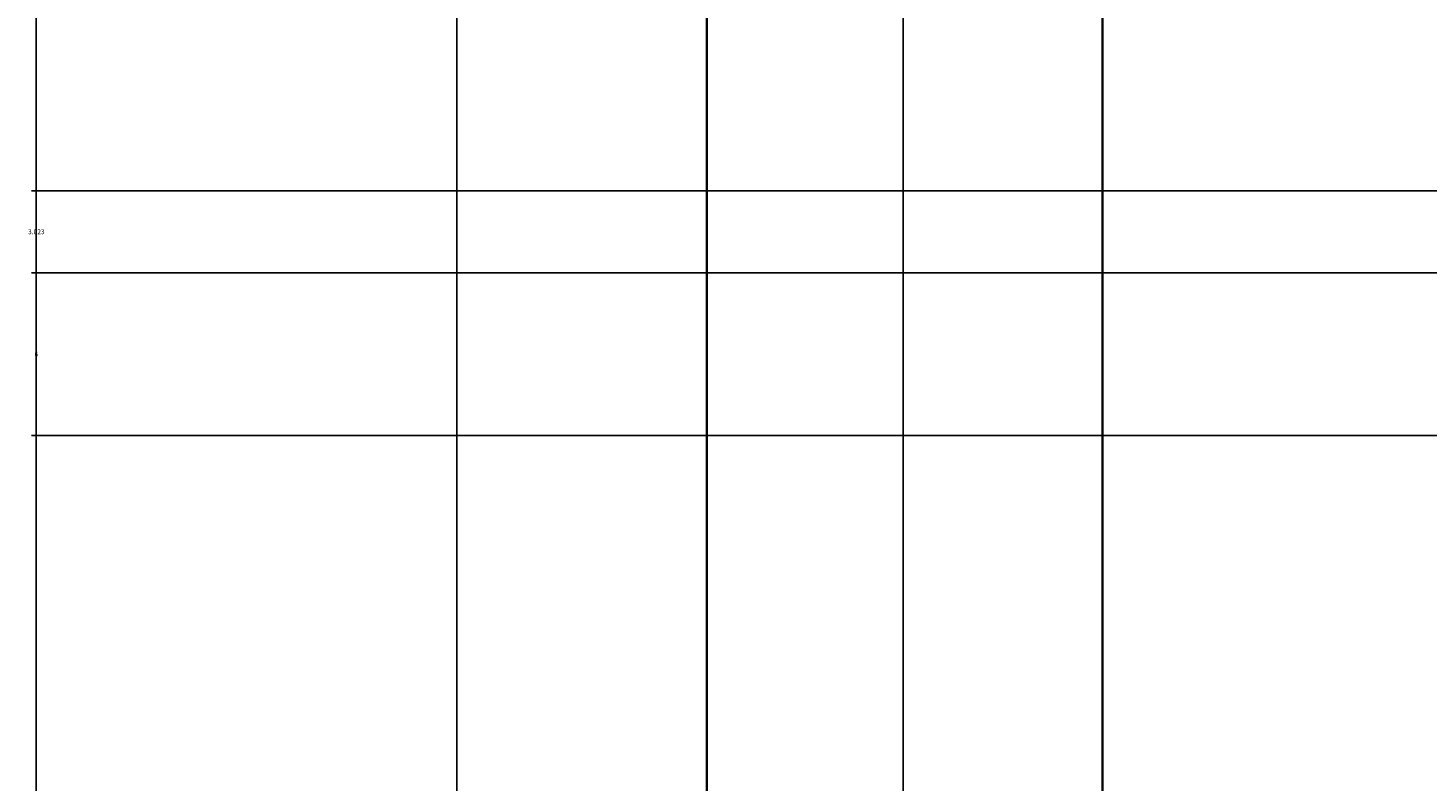
# Model space of a CAD drawing. Units: inches. Extents: x -6 to 289, y -8 to 323.
# Tile 12 of 107: x -6 to 46, y 96 to 124. Entities that reach past the tile are written whole.
import ezdxf

# ---------------------------------------------------------------- set-up
doc = ezdxf.new("R2010")
doc.units = ezdxf.units.IN
doc.header["$MEASUREMENT"] = 0
doc.layers.add('A-ANNO-DIMS', color=2, linetype='Continuous', lineweight=18)
doc.layers.add('A-ELEV', color=7, linetype='Continuous', lineweight=35)
doc.styles.get("Standard").update_dxf_attribs({"font": 'arial.ttf'})
doc.dimstyles.get("Standard").update_dxf_attribs({"dimtxt": 0.18, "dimasz": 0.18, "dimexe": 0.18, "dimexo": 0.0625, "dimgap": 0.09, "dimtad": 0, "dimtih": 1, "dimtoh": 1, "dimdec": 4, "dimzin": 0, "dimdsep": 46, "dimtxsty": 'Standard', "dimcen": 0.09, "dimadec": 0, "dimazin": 0, "dimtfac": 1, "dimtdec": 4, "dimtofl": 0, "dimtmove": 0, "dimatfit": 3, "dimfxl": 1, "dimtolj": 1, "dimtzin": 0, "dimarcsym": 0})

# ---------------------------------------------------------------- blocks, each defined once
blk = doc.blocks.new('*D19')
at = {"layer": 'A-ANNO-DIMS', "color": 0, "lineweight": -2, "transparency": 16777216}
for p, q in [((45.681, 277.043), (-5.737, 277.043)), ((-5.557, 276.863), (-5.557, 179.825)), ((-5.557, 82.423), (-5.557, 179.461)), ((45.681, 82.243), (-5.737, 82.243))]:
    blk.add_line(p, q, dxfattribs=at)
at = {"layer": 'A-ANNO-DIMS', "color": 0, "transparency": 16777216}
for points in [[(-5.587, 276.863), (-5.527, 276.863), (-5.557, 277.043)], [(-5.587, 82.423), (-5.527, 82.423), (-5.557, 82.243)]]:
    blk.add_solid(points, dxfattribs=at)
at = {"layer": 'Defpoints', "color": 0, "transparency": 16777216}
for p in [(-5.557, 277.043), (45.744, 277.043), (45.744, 82.243)]:
    blk.add_point(p, dxfattribs=at)
at = {"layer": 'A-ANNO-DIMS', "color": 0, "transparency": 16777216, "insert": (-5.557, 179.643), "char_height": 0.18, "attachment_point": 5}
blk.add_mtext('\\A1;194.8', dxfattribs=at)
blk = doc.blocks.new('*D22')
at = {"layer": 'A-ANNO-DIMS', "color": 0, "lineweight": -2, "transparency": 16777216}
for p, q in [((19.101, 307.289), (-5.737, 307.289)), ((-5.557, 307.109), (-5.557, 157.471)), ((-5.557, 7.469), (-5.557, 157.107)), ((11.907, 7.289), (-5.737, 7.289))]:
    blk.add_line(p, q, dxfattribs=at)
at = {"layer": 'A-ANNO-DIMS', "color": 0, "transparency": 16777216}
for points in [[(-5.587, 307.109), (-5.527, 307.109), (-5.557, 307.289)], [(-5.587, 7.469), (-5.527, 7.469), (-5.557, 7.289)]]:
    blk.add_solid(points, dxfattribs=at)
at = {"layer": 'Defpoints', "color": 0, "transparency": 16777216}
for p in [(19.164, 307.289), (-5.557, 7.289), (11.969, 7.289)]:
    blk.add_point(p, dxfattribs=at)
at = {"layer": 'A-ANNO-DIMS', "color": 0, "transparency": 16777216, "insert": (-5.557, 157.289), "char_height": 0.18, "attachment_point": 5}
blk.add_mtext('\\A1;300', dxfattribs=at)
blk = doc.blocks.new('*D57')
at = {"layer": 'A-ANNO-DIMS', "color": 0, "lineweight": -2, "transparency": 16777216}
for p, q in [((9.943, 68.495), (9.943, 322.969)), ((10.123, 322.789), (17.788, 322.789)), ((26.223, 322.789), (18.558, 322.789)), ((26.403, 68.495), (26.403, 322.969))]:
    blk.add_line(p, q, dxfattribs=at)
at = {"layer": 'A-ANNO-DIMS', "color": 0, "transparency": 16777216}
for points in [[(10.123, 322.819), (10.123, 322.759), (9.943, 322.789)], [(26.223, 322.819), (26.223, 322.759), (26.403, 322.789)]]:
    blk.add_solid(points, dxfattribs=at)
at = {"layer": 'Defpoints', "color": 0, "transparency": 16777216}
for p in [(26.403, 322.789), (9.943, 68.432), (26.403, 68.432)]:
    blk.add_point(p, dxfattribs=at)
at = {"layer": 'A-ANNO-DIMS', "color": 0, "transparency": 16777216, "insert": (18.173, 322.789), "char_height": 0.18, "attachment_point": 5}
blk.add_mtext('\\A1;16.46', dxfattribs=at)
blk = doc.blocks.new('*D87')
at = {"layer": 'A-ANNO-DIMS', "color": 0, "lineweight": -2, "transparency": 16777216}
for p, q in [((142.233, 108.948), (-5.737, 108.948)), ((-5.557, 108.768), (-5.557, 92.641)), ((-5.557, 76.151), (-5.557, 92.277)), ((166.233, 75.971), (-5.737, 75.971))]:
    blk.add_line(p, q, dxfattribs=at)
at = {"layer": 'A-ANNO-DIMS', "color": 0, "transparency": 16777216}
for points in [[(-5.587, 108.768), (-5.527, 108.768), (-5.557, 108.948)], [(-5.587, 76.151), (-5.527, 76.151), (-5.557, 75.971)]]:
    blk.add_solid(points, dxfattribs=at)
at = {"layer": 'Defpoints', "color": 0, "transparency": 16777216}
for p in [(-5.557, 108.948), (142.296, 108.948), (166.296, 75.971)]:
    blk.add_point(p, dxfattribs=at)
at = {"layer": 'A-ANNO-DIMS', "color": 0, "transparency": 16777216, "insert": (-5.557, 92.459), "char_height": 0.18, "attachment_point": 5}
blk.add_mtext('\\A1;32.98', dxfattribs=at)
blk = doc.blocks.new('*D88')
at = {"layer": 'A-ANNO-DIMS', "color": 0, "lineweight": -2, "transparency": 16777216}
for p, q in [((138.233, 114.948), (-5.737, 114.948)), ((-5.557, 114.768), (-5.557, 112.13)), ((-5.557, 109.128), (-5.557, 111.766)), ((142.233, 108.948), (-5.737, 108.948))]:
    blk.add_line(p, q, dxfattribs=at)
at = {"layer": 'A-ANNO-DIMS', "color": 0, "transparency": 16777216}
for points in [[(-5.587, 114.768), (-5.527, 114.768), (-5.557, 114.948)], [(-5.587, 109.128), (-5.527, 109.128), (-5.557, 108.948)]]:
    blk.add_solid(points, dxfattribs=at)
at = {"layer": 'Defpoints', "color": 0, "transparency": 16777216}
for p in [(-5.557, 114.948), (138.296, 114.948), (142.296, 108.948)]:
    blk.add_point(p, dxfattribs=at)
at = {"layer": 'A-ANNO-DIMS', "color": 0, "transparency": 16777216, "insert": (-5.557, 111.948), "char_height": 0.18, "attachment_point": 5}
blk.add_mtext('\\A1;6', dxfattribs=at)
blk = doc.blocks.new('*D89')
at = {"layer": 'A-ANNO-DIMS', "color": 0, "lineweight": -2, "transparency": 16777216}
for p, q in [((135.233, 117.971), (-5.737, 117.971)), ((-5.557, 117.791), (-5.557, 116.641)), ((-5.557, 115.128), (-5.557, 116.277)), ((138.233, 114.948), (-5.737, 114.948))]:
    blk.add_line(p, q, dxfattribs=at)
at = {"layer": 'A-ANNO-DIMS', "color": 0, "transparency": 16777216}
for points in [[(-5.587, 117.791), (-5.527, 117.791), (-5.557, 117.971)], [(-5.587, 115.128), (-5.527, 115.128), (-5.557, 114.948)]]:
    blk.add_solid(points, dxfattribs=at)
at = {"layer": 'Defpoints', "color": 0, "transparency": 16777216}
for p in [(-5.557, 117.971), (135.296, 117.971), (138.296, 114.948)]:
    blk.add_point(p, dxfattribs=at)
at = {"layer": 'A-ANNO-DIMS', "color": 0, "transparency": 16777216, "insert": (-5.557, 116.459), "char_height": 0.18, "attachment_point": 5}
blk.add_mtext('\\A1;3.023', dxfattribs=at)

msp = doc.modelspace()

# ---------------------------------------------------------------- linework, layer by layer
at = {"layer": 'A-ELEV'}
msp.add_line((19.1638, 307.2888), (19.1638, 68.4322), dxfattribs=at)
msp.add_lwpolyline([(33.7437, 289.0427), (99.7007, 289.0427), (99.7007, 70.2425), (33.7437, 70.2425)], close=True, dxfattribs=at)

# ---------------------------------------------------------------- dimensions: what is measured, and where the dimension line sits
at = {"layer": 'A-ANNO-DIMS'}
dim = msp.add_linear_dim(base=(26.403, 322.7888), p1=(9.943, 68.4322), p2=(26.403, 68.4322), dimstyle='Standard', override={"dimdec": 2, "dimlfac": 1, "dimrnd": 0, "dimzin": 0, "dimdsep": 46, "dimlunit": 2}, dxfattribs=at)
dim.commit()
dim.dimension.update_dxf_attribs({"geometry": '*D57', "text_midpoint": (18.173, 322.7888)})
for base, p1, p2, override, picture, middle in [((-5.557, 7.2888), (19.1638, 307.2888), (11.9692, 7.2888), {"dimdec": 0, "dimlfac": 1, "dimrnd": 0, "dimzin": 0, "dimdsep": 46, "dimlunit": 2}, '*D22', (-5.557, 157.2888)), ((-5.557, 277.0427), (45.7437, 82.2425), (45.7437, 277.0427), {"dimdec": 1, "dimlfac": 1, "dimrnd": 0, "dimzin": 0, "dimdsep": 46, "dimlunit": 2}, '*D19', (-5.557, 179.6426)), ((-5.557, 117.9706), (138.296, 114.9477), (135.296, 117.9706), {"dimdec": 3, "dimlfac": 1, "dimrnd": 0, "dimzin": 0, "dimdsep": 46, "dimlunit": 2}, '*D89', (-5.557, 116.4592)), ((-5.557, 114.9477), (142.296, 108.9477), (138.296, 114.9477), {"dimdec": 0, "dimlfac": 1, "dimrnd": 0, "dimzin": 0, "dimdsep": 46, "dimlunit": 2}, '*D88', (-5.557, 111.9477)), ((-5.557, 108.9477), (166.296, 75.9706), (142.296, 108.9477), {"dimdec": 2, "dimlfac": 1, "dimrnd": 0, "dimzin": 0, "dimdsep": 46, "dimlunit": 2}, '*D87', (-5.557, 92.4592))]:
    dim = msp.add_linear_dim(base=base, p1=p1, p2=p2, angle=90, dimstyle='Standard', override=override, dxfattribs=at)
    dim.commit()
    dim.dimension.update_dxf_attribs({"geometry": picture, "text_midpoint": middle})

doc.saveas('drawing.dxf')
